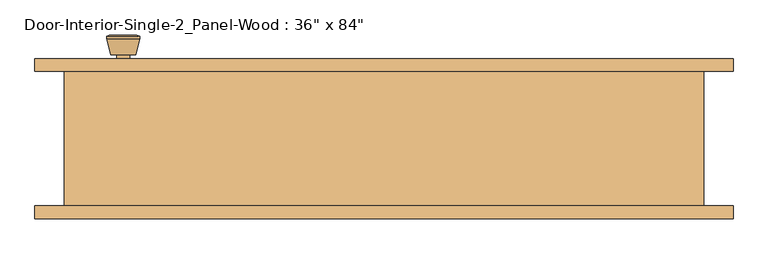
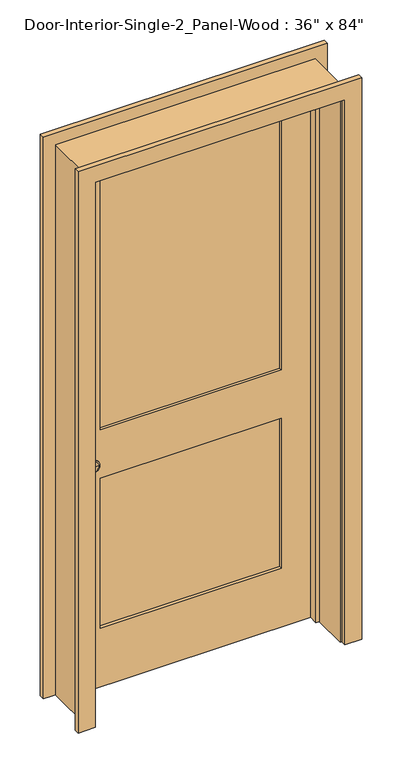
"""IFC4 building model written with IfcOpenShell, lengths in millimetres: door geometry."""

from ifc_helpers import new_model, si_unit, point, frame, frame_2d, origin, place, context, project, spatial, polyline, circle_curve, trimmed, segment, composite_curve, outline, extrude, faceted_brep, source, transform, mapped, element, save
from ifc_brep_helpers import plane_surface, cylinder_surface, revolved_surface, advanced_brep


def door_6f959a6d(model_context):
    return source(origin(), model_context, "Body", "SolidModel", [
        advanced_brep(
        [(-393.7, 57.5, 914.4), (-383.7, 57.5, 914.4), (-403.7, 57.5, 914.4), (-373.2241324, 8.5, 914.4), (-393.7, 8.5, 914.4), (-414.1758676, 8.5, 914.4), (-368.7, 10.3278681, 914.4), (-418.7, 10.3278681, 914.4), (-368.7, 13.7915463, 914.4), (-418.7, 13.7915463, 914.4), (-375.063764, 38.5, 914.4), (-412.336236, 38.5, 914.4), (-383.7, 38.5, 914.4), (-403.7, 38.5, 914.4)],
        [
            (0, 1),
            (1, 2, circle_curve(frame((-393.7, 57.5, 914.4), z_axis=(0.0, 1.0, 0.0), x_axis=(-1.0, 0.0, 0.0)), 10.0)),
            (2, 0),
            (2, 1, circle_curve(frame((-393.7, 57.5, 914.4), z_axis=(0.0, 1.0, 0.0), x_axis=(-1.0, 0.0, 0.0)), 10.0)),
            (3, 4),
            (4, 5),
            (5, 3, circle_curve(frame((-393.7, 8.5, 914.4), z_axis=(0.0, -1.0, 0.0), x_axis=(-1.0, 0.0, 0.0)), 20.4758676)),
            (3, 5, circle_curve(frame((-393.7, 8.5, 914.4), z_axis=(0.0, -1.0, 0.0), x_axis=(-1.0, 0.0, 0.0)), 20.4758676)),
            (6, 3),
            (5, 7),
            (7, 6, circle_curve(frame((-393.7, 10.3278681, 914.4), z_axis=(0.0, -1.0, 0.0), x_axis=(-1.0, 0.0, 0.0)), 25.0)),
            (6, 7, circle_curve(frame((-393.7, 10.3278681, 914.4), z_axis=(0.0, -1.0, 0.0), x_axis=(-1.0, 0.0, 0.0)), 25.0)),
            (8, 6),
            (7, 9),
            (9, 8, circle_curve(frame((-393.7, 13.7915463, 914.4), z_axis=(0.0, -1.0, 0.0), x_axis=(-1.0, 0.0, 0.0)), 25.0)),
            (8, 9, circle_curve(frame((-393.7, 13.7915463, 914.4), z_axis=(0.0, -1.0, 0.0), x_axis=(-1.0, 0.0, 0.0)), 25.0)),
            (10, 8),
            (9, 11),
            (11, 10, circle_curve(frame((-393.7, 38.5, 914.4), z_axis=(0.0, -1.0, 0.0), x_axis=(-1.0, 0.0, 0.0)), 18.636236)),
            (10, 11, circle_curve(frame((-393.7, 38.5, 914.4), z_axis=(0.0, -1.0, 0.0), x_axis=(-1.0, 0.0, 0.0)), 18.636236)),
            (12, 10),
            (11, 13),
            (13, 12, circle_curve(frame((-393.7, 38.5, 914.4), z_axis=(0.0, -1.0, 0.0), x_axis=(-1.0, 0.0, 0.0)), 10.0)),
            (12, 13, circle_curve(frame((-393.7, 38.5, 914.4), z_axis=(0.0, -1.0, 0.0), x_axis=(-1.0, 0.0, 0.0)), 10.0)),
            (1, 12),
            (13, 2),
        ],
        [
            plane_surface(frame((-393.7, 57.5, 914.4), z_axis=(0.0, 1.0, 0.0), x_axis=(-1.0, 0.0, 0.0))),
            plane_surface(frame((-393.7, 8.5, 914.4), z_axis=(0.0, -1.0, 0.0), x_axis=(-1.0, 0.0, 0.0))),
            revolved_surface(polyline([(-414.1758676, 8.5, 914.4), (-418.7, 10.3278681, 914.4)]), (-393.7, 57.5, 914.4), (0.0, 1.0, 0.0)),
            cylinder_surface(frame((-393.7, 57.5, 914.4), z_axis=(0.0, 1.0, 0.0), x_axis=(-1.0, 0.0, 0.0)), 25.0),
            revolved_surface(polyline([(-418.7, 13.7915463, 914.4), (-412.336236, 38.5, 914.4)]), (-393.7, 57.5, 914.4), (0.0, 1.0, 0.0)),
            plane_surface(frame((-393.7, 38.5, 914.4), z_axis=(0.0, 1.0, 0.0), x_axis=(-1.0, 0.0, 0.0))),
            cylinder_surface(frame((-393.7, 57.5, 914.4), z_axis=(0.0, 1.0, 0.0), x_axis=(-1.0, 0.0, 0.0)), 10.0),
        ],
        [
            (0, [[1, 2, 3]]),
            (0, [[-3, 4, -1]]),
            (1, [[5, 6, 7]]),
            (1, [[-6, -5, 8]]),
            (2, [[9, -7, 10, 11]]),
            (2, [[-10, -8, -9, 12]]),
            (3, [[13, -11, 14, 15]]),
            (3, [[-14, -12, -13, 16]]),
            (4, [[17, -15, 18, 19]]),
            (4, [[-18, -16, -17, 20]]),
            (5, [[21, -19, 22, 23]]),
            (5, [[-22, -20, -21, 24]]),
            (6, [[25, -23, 26, -2]]),
            (6, [[-26, -24, -25, -4]]),
        ],
    ),
        extrude(outline(composite_curve([segment(trimmed(circle_curve(frame_2d((914.4, -393.7)), 30.0), [point((914.4, -423.7))], [point((914.4, -363.7))], False, "CARTESIAN"), True, "CONTINUOUS"), segment(trimmed(circle_curve(frame_2d((914.4, -393.7)), 30.0), [point((914.4, -363.7))], [point((914.4, -423.7))], False, "CARTESIAN"), True, "CONTINUOUS")], self_intersect=False)), frame((0.0, 57.5, 0.0), z_axis=(0.0, 1.0, 0.0), x_axis=(0.0, 0.0, 1.0)), (0.0, 0.0, 1.0), 6.0),
        advanced_brep(
        [(-393.7, 104.425, 914.4), (-403.7, 104.425, 914.4), (-383.7, 104.425, 914.4), (-373.2241324, 153.425, 914.4), (-414.1758676, 153.425, 914.4), (-393.7, 153.425, 914.4), (-368.7, 151.5971319, 914.4), (-418.7, 151.5971319, 914.4), (-368.7, 148.1334537, 914.4), (-418.7, 148.1334537, 914.4), (-375.063764, 123.425, 914.4), (-412.336236, 123.425, 914.4), (-383.7, 123.425, 914.4), (-403.7, 123.425, 914.4)],
        [
            (0, 1),
            (1, 2, circle_curve(frame((-393.7, 104.425, 914.4), z_axis=(0.0, -1.0, 0.0), x_axis=(-1.0, 0.0, 0.0)), 10.0)),
            (2, 0),
            (2, 1, circle_curve(frame((-393.7, 104.425, 914.4), z_axis=(0.0, -1.0, 0.0), x_axis=(-1.0, 0.0, 0.0)), 10.0)),
            (3, 4, circle_curve(frame((-393.7, 153.425, 914.4), z_axis=(0.0, 1.0, 0.0), x_axis=(-1.0, 0.0, 0.0)), 20.4758676)),
            (4, 5),
            (5, 3),
            (4, 3, circle_curve(frame((-393.7, 153.425, 914.4), z_axis=(0.0, 1.0, 0.0), x_axis=(-1.0, 0.0, 0.0)), 20.4758676)),
            (6, 7, circle_curve(frame((-393.7, 151.5971319, 914.4), z_axis=(0.0, 1.0, 0.0), x_axis=(-1.0, 0.0, 0.0)), 25.0)),
            (7, 4),
            (3, 6),
            (7, 6, circle_curve(frame((-393.7, 151.5971319, 914.4), z_axis=(0.0, 1.0, 0.0), x_axis=(-1.0, 0.0, 0.0)), 25.0)),
            (8, 9, circle_curve(frame((-393.7, 148.1334537, 914.4), z_axis=(0.0, 1.0, 0.0), x_axis=(-1.0, 0.0, 0.0)), 25.0)),
            (9, 7),
            (6, 8),
            (9, 8, circle_curve(frame((-393.7, 148.1334537, 914.4), z_axis=(0.0, 1.0, 0.0), x_axis=(-1.0, 0.0, 0.0)), 25.0)),
            (10, 11, circle_curve(frame((-393.7, 123.425, 914.4), z_axis=(0.0, 1.0, 0.0), x_axis=(-1.0, 0.0, 0.0)), 18.636236)),
            (11, 9),
            (8, 10),
            (11, 10, circle_curve(frame((-393.7, 123.425, 914.4), z_axis=(0.0, 1.0, 0.0), x_axis=(-1.0, 0.0, 0.0)), 18.636236)),
            (12, 13, circle_curve(frame((-393.7, 123.425, 914.4), z_axis=(0.0, 1.0, 0.0), x_axis=(-1.0, 0.0, 0.0)), 10.0)),
            (13, 11),
            (10, 12),
            (13, 12, circle_curve(frame((-393.7, 123.425, 914.4), z_axis=(0.0, 1.0, 0.0), x_axis=(-1.0, 0.0, 0.0)), 10.0)),
            (1, 13),
            (12, 2),
        ],
        [
            plane_surface(frame((-393.7, 104.425, 914.4), z_axis=(0.0, -1.0, 0.0), x_axis=(-1.0, 0.0, 0.0))),
            plane_surface(frame((-393.7, 153.425, 914.4), z_axis=(0.0, 1.0, 0.0), x_axis=(-1.0, 0.0, 0.0))),
            revolved_surface(polyline([(-414.1758676, 153.425, 914.4), (-418.7, 151.5971319, 914.4)]), (-393.7, 104.425, 914.4), (0.0, -1.0, 0.0)),
            cylinder_surface(frame((-393.7, 104.425, 914.4), z_axis=(0.0, -1.0, 0.0), x_axis=(-1.0, 0.0, 0.0)), 25.0),
            revolved_surface(polyline([(-418.7, 148.1334537, 914.4), (-412.336236, 123.425, 914.4)]), (-393.7, 104.425, 914.4), (0.0, -1.0, 0.0)),
            plane_surface(frame((-393.7, 123.425, 914.4), z_axis=(0.0, -1.0, 0.0), x_axis=(-1.0, 0.0, 0.0))),
            cylinder_surface(frame((-393.7, 104.425, 914.4), z_axis=(0.0, -1.0, 0.0), x_axis=(-1.0, 0.0, 0.0)), 10.0),
        ],
        [
            (0, [[1, 2, 3]]),
            (0, [[-3, 4, -1]]),
            (1, [[5, 6, 7]]),
            (1, [[8, -7, -6]]),
            (2, [[9, 10, -5, 11]]),
            (2, [[12, -11, -8, -10]]),
            (3, [[13, 14, -9, 15]]),
            (3, [[16, -15, -12, -14]]),
            (4, [[17, 18, -13, 19]]),
            (4, [[20, -19, -16, -18]]),
            (5, [[21, 22, -17, 23]]),
            (5, [[24, -23, -20, -22]]),
            (6, [[-2, 25, -21, 26]]),
            (6, [[-4, -26, -24, -25]]),
        ],
    ),
        extrude(outline(composite_curve([segment(trimmed(circle_curve(frame_2d((914.4, -393.7)), 30.0), [point((914.4, -423.7))], [point((914.4, -363.7))], False, "CARTESIAN"), True, "CONTINUOUS"), segment(trimmed(circle_curve(frame_2d((914.4, -393.7)), 30.0), [point((914.4, -363.7))], [point((914.4, -423.7))], False, "CARTESIAN"), True, "CONTINUOUS")], self_intersect=False)), frame((0.0, 98.425, 0.0), z_axis=(0.0, 1.0, 0.0), x_axis=(0.0, 0.0, 1.0)), (0.0, 0.0, 1.0), 6.0),
        extrude(outline(polyline([(336.55, 75.1416667), (-336.55, 75.1416667), (-336.55, 86.7833333), (336.55, 86.7833333), (336.55, 75.1416667)])), frame((0.0, 0.0, 1009.65), z_axis=(0.0, 0.0, 1.0), x_axis=(1.0, 0.0, 0.0)), (0.0, 0.0, 1.0), 1004.8875),
        extrude(outline(polyline([(336.55, 75.1416667), (-336.55, 75.1416667), (-336.55, 86.7833333), (336.55, 86.7833333), (336.55, 75.1416667)])), frame((0.0, 0.0, 231.775), z_axis=(0.0, 0.0, 1.0), x_axis=(1.0, 0.0, 0.0)), (0.0, 0.0, 1.0), 587.375),
        extrude(outline(polyline([(2133.6, -457.2), (0.0, -457.2), (0.0, 457.2), (2133.6, 457.2), (2133.6, -457.2)]), holes=[polyline([(2014.5375, -336.55), (2014.5375, 336.55), (1009.65, 336.55), (1009.65, -336.55), (2014.5375, -336.55)]), polyline([(819.15, -336.55), (819.15, 336.55), (231.775, 336.55), (231.775, -336.55), (819.15, -336.55)])]), frame((0.0, 63.5, 0.0), z_axis=(0.0, 1.0, 0.0), x_axis=(0.0, 0.0, 1.0)), (0.0, 0.0, 1.0), 34.925),
        faceted_brep([(482.6, 98.425, 0.0), (482.6, -104.775, 0.0), (457.2, -104.775, 0.0), (457.2, 28.575, 0.0), (444.5, 28.575, 0.0), (444.5, 63.5, 0.0), (457.2, 63.5, 0.0), (457.2, 98.425, 0.0), (482.6, 98.425, 2159.0), (482.6, -104.775, 2159.0), (-482.6, -104.775, 2159.0), (-482.6, -104.775, 0.0), (-457.2, -104.775, 0.0), (-457.2, -104.775, 2133.6), (457.2, -104.775, 2133.6), (457.2, 28.575, 2133.6), (-457.2, 28.575, 2133.6), (-457.2, 28.575, 0.0), (-444.5, 28.575, 0.0), (-444.5, 28.575, 2120.9), (444.5, 28.575, 2120.9), (444.5, 63.5, 2120.9), (-444.5, 63.5, 2120.9), (-444.5, 63.5, 0.0), (-457.2, 63.5, 0.0), (-457.2, 63.5, 2133.6), (457.2, 63.5, 2133.6), (457.2, 98.425, 2133.6), (-457.2, 98.425, 2133.6), (-457.2, 98.425, 0.0), (-482.6, 98.425, 0.0), (-482.6, 98.425, 2159.0)], [[[0, 1, 2, 3, 4, 5, 6, 7]], [[1, 0, 8, 9]], [[2, 1, 9, 10, 11, 12, 13, 14]], [[3, 2, 14, 15]], [[4, 3, 15, 16, 17, 18, 19, 20]], [[5, 4, 20, 21]], [[6, 5, 21, 22, 23, 24, 25, 26]], [[7, 6, 26, 27]], [[0, 7, 27, 28, 29, 30, 31, 8]], [[9, 8, 31, 10]], [[15, 14, 13, 16]], [[21, 20, 19, 22]], [[27, 26, 25, 28]], [[30, 29, 24, 23, 18, 17, 12, 11]], [[10, 31, 30, 11]], [[16, 13, 12, 17]], [[22, 19, 18, 23]], [[28, 25, 24, 29]]]),
        extrude(outline(polyline([(0.0, 463.55), (0.0, 527.05), (2203.45, 527.05), (2203.45, -527.05), (0.0, -527.05), (0.0, -463.55), (2139.95, -463.55), (2139.95, 463.55), (0.0, 463.55)])), frame((0.0, -123.825, 0.0), z_axis=(0.0, 1.0, 0.0), x_axis=(0.0, 0.0, 1.0)), (0.0, 0.0, 1.0), 19.05),
        extrude(outline(polyline([(0.0, 463.55), (0.0, 527.05), (2203.45, 527.05), (2203.45, -527.05), (0.0, -527.05), (0.0, -463.55), (2139.95, -463.55), (2139.95, 463.55), (0.0, 463.55)])), frame((0.0, 98.425, 0.0), z_axis=(0.0, 1.0, 0.0), x_axis=(0.0, 0.0, 1.0)), (0.0, 0.0, 1.0), 19.05),
    ])


if __name__ == "__main__":
    model = new_model("IFC4")
    model_context = context("Model", 3, world=origin())
    ifc_project = project(units=[si_unit("LENGTHUNIT", "METRE", prefix="MILLI")], contexts=[model_context])
    site = spatial("IfcSite", under=ifc_project)
    building = spatial("IfcBuilding", under=site)
    placement = place(None, origin())
    door_shape = door_6f959a6d(model_context)
    element("IfcDoor", 1, ObjectType="Door-Interior-Single-2_Panel-Wood : 36\" x 84\"", at=placement, inside=building, context=model_context, shape_type="MappedRepresentation", body=[
        mapped(door_shape, transform((0.0, 0.0, 0.0), x_axis=(1.0, 0.0, 0.0), y_axis=(0.0, 1.0, 0.0), z_axis=(0.0, 0.0, 1.0))),
    ])
    save(model, "model.ifc")

# Revit data of these elements
# Type "Door-Interior-Single-2_Panel-Wood : 36\" x 84\""
#   Type Mark = "9"
#   Assembly Code = "C1020300"
#   Analytic Construction = "Wooden"
#   Top Rail = 0' - 4 11/16"
#   Thickness = 0' - 1 3/8"
#   Thermal Resistance (R) = 2.5876 (h·ft²·°F)/BTU
#   Swing Angle [instance default] = 90.00°
#   Stiles = 0' - 4 3/4"
#   Rough Width = 3' - 2"
#   Rough Height = 7' - 1"
#   Lock Rail = 0' - 7 1/2"
#   Height = 7' - 0"
#   Width = 3' - 0"
#   Heat Transfer Coefficient (U) = 0.3865 BTU/(h·ft²·°F)
#   Bottom Rail = 0' - 9 1/8"
#   Trim Material = Cherry
#   Panel Material = Cherry
#   Frame Material = Cherry
#   Door Handle Material = Aluminum
#   Visual Light Transmittance = 0
#   Solar Heat Gain Coefficient = 0
#   Wall Closure = (empty or 0)
#   Function = (empty or 0)
# Element 1 (IfcDoor, "Door-Interior-Single-2_Panel-Wood : 36\" x 84\"")
#   Materials on its faces: "Cherry", "Aluminum"
# Materials
#   "Cherry": class "Wood", colour RGB 226 177 128, transparency 0, Description = "Prunus Serotina", Cost = 0
#   "Aluminum": class "Metal", colour RGB 247 247 247, transparency 0, Description = "Aluminum 6061", Cost = 0
